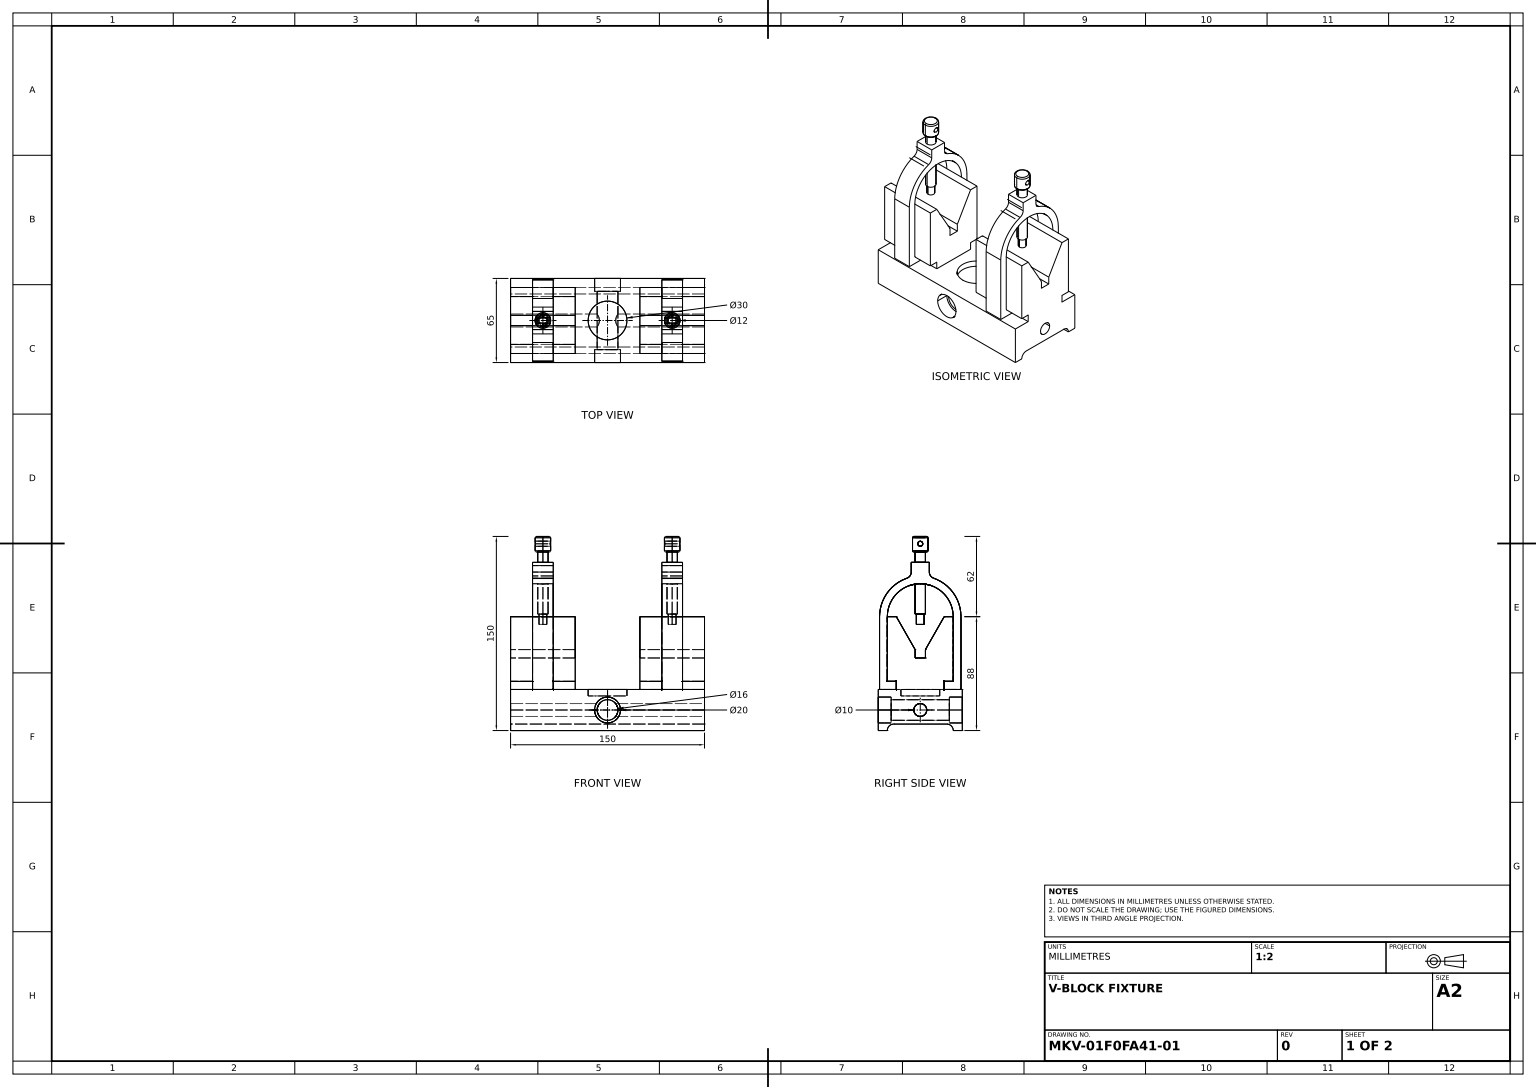
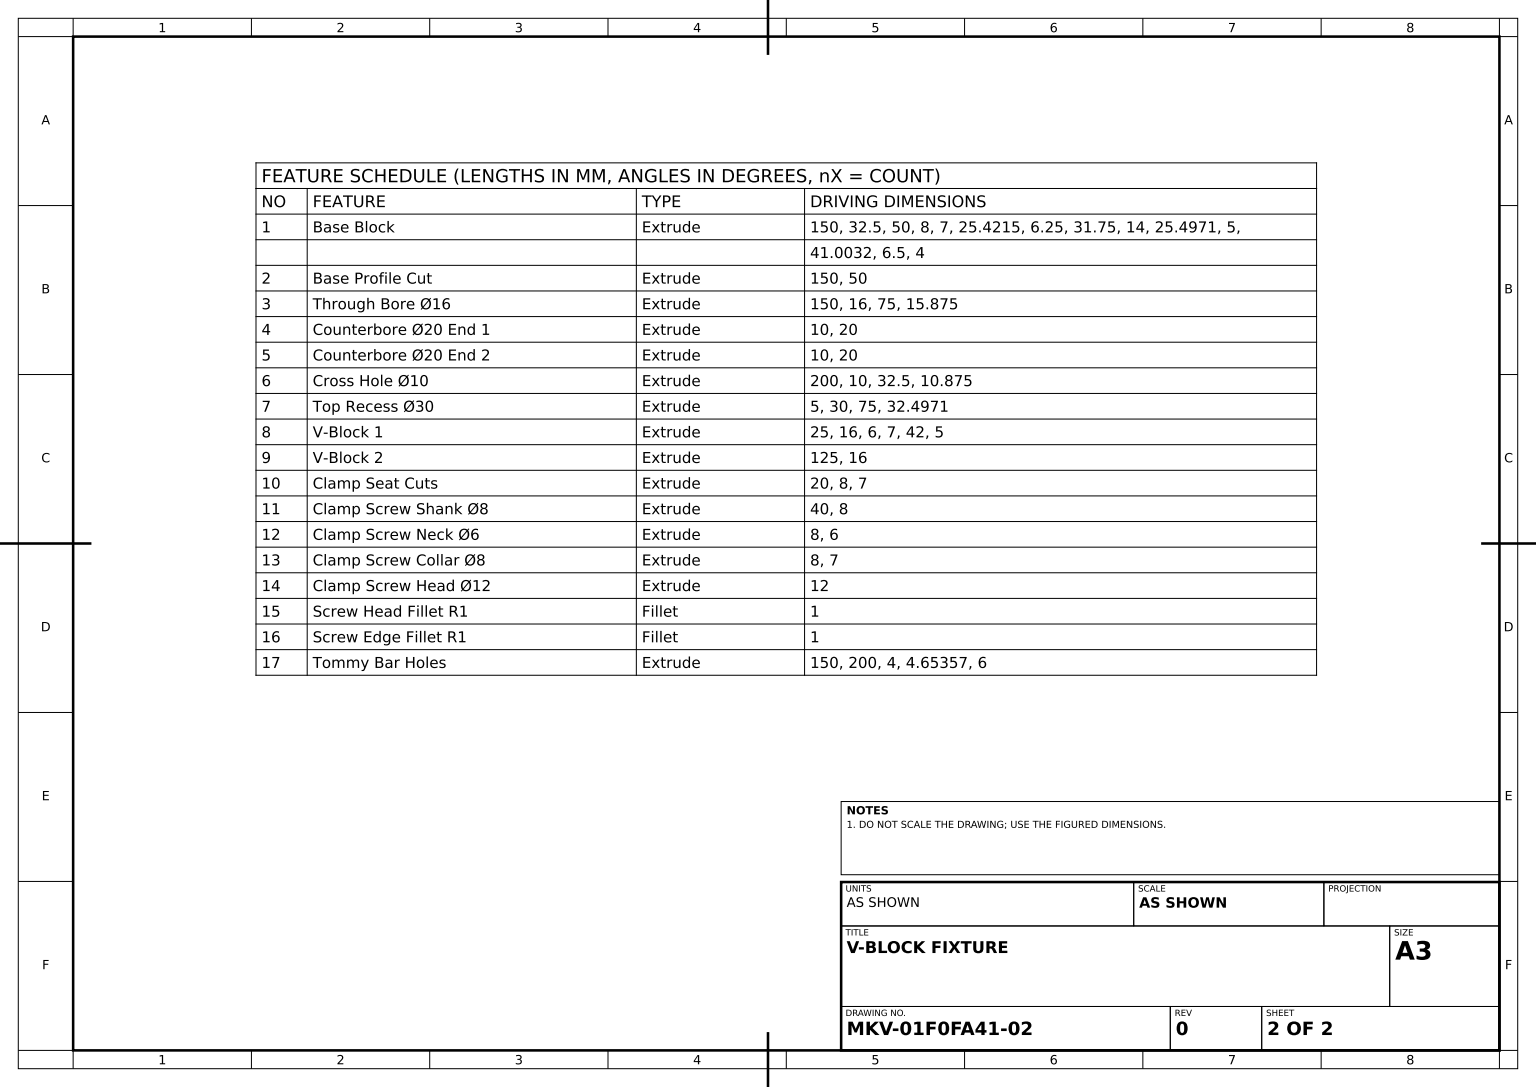
from build123d import *

# Parameters (mm, degrees)
BASE_BLOCK_DEPTH            = 150
BASE_PROFILE_CUT_SKETCH_W   = 50
BASE_PROFILE_CUT_SKETCH_H   = 50
BASE_PROFILE_CUT_SKETCH_H_2 = 6.25
BASE_PROFILE_CUT_DEPTH      = 150
THROUGH_BORE_SKETCH_R       = 8
THROUGH_BORE_16_DEPTH       = 150
COUNTERBORE_END_1_SKETCH_R  = 10
COUNTERBORE_20_END_1_DEPTH  = 10
COUNTERBORE_START           = -10
COUNTERBORE_END_2_SKETCH_R  = 10
COUNTERBORE_20_END_2_DEPTH  = 10
CROSS_HOLE_SKETCH_R         = 5
CROSS_HOLE_10_DEPTH         = 200
TOP_RECESS_SKETCH_R         = 15
TOP_RECESS_30_DEPTH         = 5
V_BLOCK_1_DEPTH             = 8
V_BLOCK_2_DEPTH             = 8
CLAMP_SEAT_CUT_SKETCH_R     = 4
CLAMP_SEAT_CUTS_DEPTH       = 20
CLAMP_SCREW_SHANK_SKETCH_R  = 4
CLAMP_SCREW_SHANK_8_DEPTH   = 40
CLAMP_SCREW_NECK_SKETCH_R   = 3
CLAMP_SCREW_NECK_6_DEPTH    = 8
CLAMP_START                 = 8
CLAMP_SCREW_COLLAR_SKETCH_R = 4
CLAMP_SCREW_COLLAR_8_DEPTH  = 8
CLAMP_SCREW_HEAD_SKETCH_R   = 6
CLAMP_SCREW_HEAD_12_DEPTH   = 12
SCREW_HEAD_FILLET_R1_R      = 1
SCREW_EDGE_FILLET_R1_R      = 1
TOMMY_BAR_HOLE_SKETCH_R     = 2
TOMMY_BAR_HOLES_DEPTH       = 200


with BuildPart() as part:
    # Base Block Profile Sketch → Base Block (new body)
    with BuildSketch(Plane(origin=(0, 0, 0), x_dir=(0, 0, -1), z_dir=(1, 0, 0))):
        with BuildLine():
            Line((-32.5, 0), (-25.500000237, 0))
            ThreePointArc((-25.500000237, 0), (-24.035534143, 3.535533906), (-20.500000237, 5))
            Line((-20.500000237, 5), (20.503245082, 5))
            ThreePointArc((20.503245082, 5), (24.038778988, 3.535533906), (25.503245082, 0))
            Line((25.503245082, 0), (32.5, 0))
            Line((32.5, 0), (32.5, 31.75))
            Line((32.5, 31.75), (18.5, 31.75))
            Line((18.5, 31.75), (18.5, 38))
            Line((18.5, 38), (25.5, 38))
            Line((25.5, 38), (25.5, 88))
            Line((25.5, 88), (18.5, 88))
            Line((18.5, 88), (4.002919757, 62.578494059))
            Line((4.002919757, 62.578494059), (4.002919757, 56.078494059))
            Line((4.002919757, 56.078494059), (-3.997080243, 56.078494059))
            Line((-3.997080243, 56.078494059), (-3.997080243, 62.578494059))
            Line((-3.997080243, 62.578494059), (-18.5, 88))
            Line((-18.5, 88), (-25.5, 88))
            Line((-25.5, 88), (-25.5, 38))
            Line((-25.5, 38), (-18.5, 38))
            Line((-18.5, 38), (-18.5, 31.75))
            Line((-18.5, 31.75), (-32.5, 31.75))
            Line((-32.5, 31.75), (-32.5, 0))
        make_face()
    extrude(amount=BASE_BLOCK_DEPTH)

    # Base Profile Cut Sketch → Base Profile Cut (cut)
    with BuildSketch(Plane.XY.offset(25.5)):
        with Locations((75, 63)):
            Rectangle(BASE_PROFILE_CUT_SKETCH_W, BASE_PROFILE_CUT_SKETCH_H)
        with Locations((75, 34.875)):
            Rectangle(BASE_PROFILE_CUT_SKETCH_W, BASE_PROFILE_CUT_SKETCH_H_2)
    extrude(amount=-BASE_PROFILE_CUT_DEPTH, mode=Mode.SUBTRACT)

    # Through Bore Sketch → Through Bore _16 (cut)
    with BuildSketch(Plane.XY.offset(32.5)):
        with Locations((75, 15.875)):
            Circle(THROUGH_BORE_SKETCH_R)
    extrude(amount=-THROUGH_BORE_16_DEPTH, mode=Mode.SUBTRACT)

    # Counterbore End 1 Sketch → Counterbore _20 End 1 (cut)
    with BuildSketch(Plane.XY.offset(32.5)):
        with Locations((75, 15.875)):
            Circle(COUNTERBORE_END_1_SKETCH_R)
    extrude(amount=-COUNTERBORE_20_END_1_DEPTH, mode=Mode.SUBTRACT)

    # Counterbore End 2 Sketch → Counterbore _20 End 2 (cut)
    with BuildSketch(Plane(origin=(0, 0, -32.5), x_dir=(-1, 0, 0), z_dir=(0, 0, -1)).offset(COUNTERBORE_START)):
        with Locations(Location((-75, 15.875, 0), (0, 0, 180))):
            Circle(COUNTERBORE_END_2_SKETCH_R)
    extrude(amount=COUNTERBORE_20_END_2_DEPTH, mode=Mode.SUBTRACT)

    # Cross Hole Sketch → Cross Hole _10 (cut)
    with BuildSketch(Plane.ZY):
        with Locations((0, 15.875)):
            Circle(CROSS_HOLE_SKETCH_R)
    extrude(amount=-CROSS_HOLE_10_DEPTH, mode=Mode.SUBTRACT)

    # Top Recess Sketch → Top Recess _30 (cut)
    with BuildSketch(Plane(origin=(0, 31.75, 0), x_dir=(1, 0, 0), z_dir=(0, 1, 0))):
        with Locations(Location((75, 0.002919757, 0), (0, 0, 270))):
            Circle(TOP_RECESS_SKETCH_R)
    extrude(amount=-TOP_RECESS_30_DEPTH, mode=Mode.SUBTRACT)

    # V-Block 1 Sketch → V-Block 1 (add, symmetric)
    with BuildSketch(Plane(origin=(25, 0, 0), x_dir=(0, 0, -1), z_dir=(1, 0, 0))):
        with BuildLine():
            Line((18.5, 38), (18.5, 31.75))
            Line((18.5, 31.75), (31.5, 31.75))
            Line((31.5, 31.75), (31.5, 88))
            ThreePointArc((31.5, 88), (25.675564045, 106.248709844), (10.356164384, 117.748947196))
            ThreePointArc((10.356164384, 117.748947196), (7.924513644, 119.574381696), (7, 122.471002306))
            Line((7, 122.471002306), (7, 130))
            Line((7, 130), (-7, 130))
            Line((-7, 130), (-7, 122.471002306))
            ThreePointArc((-7, 122.471002306), (-7.924513644, 119.574381696), (-10.356164384, 117.748947196))
            ThreePointArc((-10.356164384, 117.748947196), (-25.675564045, 106.248709844), (-31.5, 88))
            Line((-31.5, 88), (-31.5, 31.75))
            Line((-31.5, 31.75), (-18.5, 31.75))
            Line((-18.5, 31.75), (-18.5, 38))
            Line((-18.5, 38), (-25.5, 38))
            Line((-25.5, 38), (-25.5, 88))
            ThreePointArc((-25.5, 88), (0, 113.5), (25.5, 88))
            Line((25.5, 88), (25.5, 38))
            Line((25.5, 38), (18.5, 38))
        make_face()
    extrude(amount=V_BLOCK_1_DEPTH, both=True)

    # V-Block 2 Sketch → V-Block 2 (add, symmetric)
    with BuildSketch(Plane(origin=(125, 0, 0), x_dir=(0, 0, -1), z_dir=(1, 0, 0))):
        with BuildLine():
            Line((-31.5, 88), (-31.5, 31.75))
            Line((-31.5, 31.75), (-18.5, 31.75))
            Line((-18.5, 31.75), (-18.5, 38))
            Line((-18.5, 38), (-25.5, 38))
            Line((-25.5, 38), (-25.5, 88))
            ThreePointArc((-25.5, 88), (0, 113.5), (25.5, 88))
            Line((25.5, 88), (25.5, 38))
            Line((25.5, 38), (18.5, 38))
            Line((18.5, 38), (18.5, 31.75))
            Line((18.5, 31.75), (31.5, 31.75))
            Line((31.5, 31.75), (31.5, 88))
            ThreePointArc((31.5, 88), (25.675564045, 106.248709844), (10.356164384, 117.748947196))
            ThreePointArc((10.356164384, 117.748947196), (7.924513644, 119.574381696), (7, 122.471002306))
            Line((7, 122.471002306), (7, 130))
            Line((7, 130), (-7, 130))
            Line((-7, 130), (-7, 122.471002306))
            ThreePointArc((-7, 122.471002306), (-7.924513644, 119.574381696), (-10.356164384, 117.748947196))
            ThreePointArc((-10.356164384, 117.748947196), (-25.675564045, 106.248709844), (-31.5, 88))
        make_face()
    extrude(amount=V_BLOCK_2_DEPTH, both=True)

    # Clamp Seat Cut Sketch → Clamp Seat Cuts (cut)
    with BuildSketch(Plane(origin=(0, 130, 0), x_dir=(1, 0, 0), z_dir=(0, 1, 0))):
        with Locations(Location((25, 0, 0), (0, 0, 270))):
            Circle(CLAMP_SEAT_CUT_SKETCH_R)
        with Locations(Location((125, 0, 0), (0, 0, 270))):
            Circle(CLAMP_SEAT_CUT_SKETCH_R)
    extrude(amount=-CLAMP_SEAT_CUTS_DEPTH, mode=Mode.SUBTRACT)

    # Clamp Screw Shank Sketch → Clamp Screw Shank _8 (add)
    with BuildSketch(Plane(origin=(0, 130, 0), x_dir=(1, 0, 0), z_dir=(0, 1, 0))):
        with Locations(Location((25, 0, 0), (0, 0, 270))):
            Circle(CLAMP_SCREW_SHANK_SKETCH_R)
        with Locations(Location((125, 0, 0), (0, 0, 270))):
            Circle(CLAMP_SCREW_SHANK_SKETCH_R)
    extrude(amount=-CLAMP_SCREW_SHANK_8_DEPTH)

    # Clamp Screw Neck Sketch → Clamp Screw Neck _6 (add)
    with BuildSketch(Plane.XZ.offset(-90)):
        with Locations(Location((125, 0, 0), (0, 0, 270))):
            Circle(CLAMP_SCREW_NECK_SKETCH_R)
        with Locations(Location((25, 0, 0), (0, 0, 270))):
            Circle(CLAMP_SCREW_NECK_SKETCH_R)
    extrude(amount=CLAMP_SCREW_NECK_6_DEPTH)

    # Clamp Screw Collar Sketch → Clamp Screw Collar _8 (add)
    with BuildSketch(Plane(origin=(0, 130, 0), x_dir=(1, 0, 0), z_dir=(0, 1, 0)).offset(CLAMP_START)):
        with Locations(Location((25, 0, 0), (0, 0, 270))):
            Circle(CLAMP_SCREW_COLLAR_SKETCH_R)
        with Locations(Location((125, 0, 0), (0, 0, 270))):
            Circle(CLAMP_SCREW_COLLAR_SKETCH_R)
    extrude(amount=-CLAMP_SCREW_COLLAR_8_DEPTH)

    # Clamp Screw Head Sketch → Clamp Screw Head _12 (add)
    with BuildSketch(Plane(origin=(0, 138, 0), x_dir=(1, 0, 0), z_dir=(0, 1, 0))):
        with Locations(Location((25, 0, 0), (0, 0, 270))):
            Circle(CLAMP_SCREW_HEAD_SKETCH_R)
        with Locations(Location((125, 0, 0), (0, 0, 270))):
            Circle(CLAMP_SCREW_HEAD_SKETCH_R)
    extrude(amount=CLAMP_SCREW_HEAD_12_DEPTH)

    # Screw Head Fillet R1
    screw_head_fillet_r1_edges = [part.edges().sort_by_distance(p)[0] for p in [
        (25, 150, -6),
        (125, 150, -6),
    ]]
    fillet(screw_head_fillet_r1_edges, radius=SCREW_HEAD_FILLET_R1_R)

    # Screw Edge Fillet R1
    screw_edge_fillet_r1_edges = [part.edges().sort_by_distance(p)[0] for p in [
        (25, 138, -6),
        (125, 138, -6),
    ]]
    fillet(screw_edge_fillet_r1_edges, radius=SCREW_EDGE_FILLET_R1_R)

    # Tommy Bar Hole Sketch → Tommy Bar Holes (cut)
    with BuildSketch(Plane(origin=(150, 0, 0), x_dir=(0, 0, -1), z_dir=(1, 0, 0))):
        with Locations((0, 144.346433509)):
            Circle(TOMMY_BAR_HOLE_SKETCH_R)
    extrude(amount=-TOMMY_BAR_HOLES_DEPTH, mode=Mode.SUBTRACT)


solid = part.part
